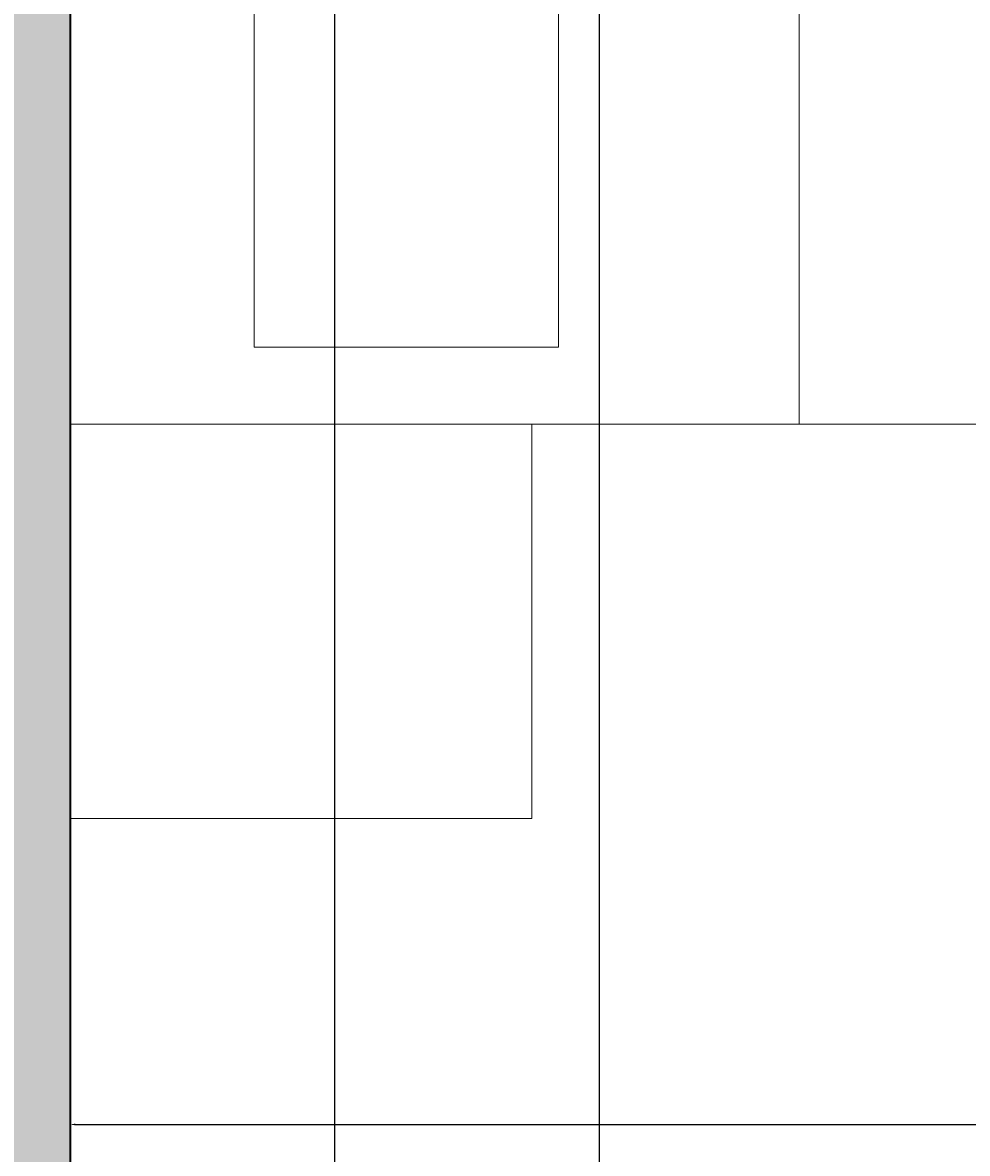
# Model space of a CAD drawing. Units: inches. Extents: x 1998 to 2588, y 1139 to 1977.
# Tile 64 of 134: x 2095 to 2127, y 1779 to 1817. Entities that reach past the tile are written whole.
import ezdxf

# ---------------------------------------------------------------- set-up
doc = ezdxf.new("R2010")
doc.units = ezdxf.units.IN
for name, color, linetype, lineweight in [('A-ANNO-DIMS', 2, 'Continuous', 18), ('A-WALL-PATT', 252, 'Continuous', 13), ('FUR', 21, 'Continuous', 18), ('WALL', 200, 'Continuous', 35)]:
    doc.layers.add(name, color=color, linetype=linetype, lineweight=lineweight)
doc.styles.get("Standard").update_dxf_attribs({"font": 'arial.ttf'})
doc.dimstyles.get("Standard").update_dxf_attribs({"dimtxt": 0.18, "dimasz": 0.18, "dimexe": 0.18, "dimexo": 0.0625, "dimgap": 0.09, "dimtad": 0, "dimtih": 1, "dimtoh": 1, "dimdec": 4, "dimzin": 0, "dimdsep": 46, "dimtxsty": 'Standard', "dimcen": 0.09, "dimadec": 0, "dimazin": 0, "dimtfac": 1, "dimtdec": 4, "dimtofl": 0, "dimtmove": 0, "dimatfit": 3, "dimfxl": 1, "dimtolj": 1, "dimtzin": 0, "dimarcsym": 0})

# ---------------------------------------------------------------- blocks, each defined once
blk = doc.blocks.new('BED-WITH-NIGHTSTANDS')
blk.add_line((24.799, 13.424), (24.799, 47.436))
for points in [[(0, 56), (65.221, 56), (65.221, 13.424), (0, 13.424)], [(6.254, 16.049), (16.605, 16.049), (16.605, 34.569), (6.254, 34.569)], [(0, 0), (15.699, 0), (15.699, 13.424), (0, 13.424)]]:
    blk.add_lwpolyline(points, close=True)
blk = doc.blocks.new('*D14')
at = {"layer": 'A-ANNO-DIMS', "color": 0, "lineweight": -2, "transparency": 16777216}
for p, q in [((2096.973, 1789.982), (2096.973, 1779.451)), ((2162.194, 1789.982), (2162.194, 1779.451)), ((2097.153, 1779.631), (2129.055, 1779.631)), ((2162.014, 1779.631), (2130.112, 1779.631))]:
    blk.add_line(p, q, dxfattribs=at)
at = {"layer": 'A-ANNO-DIMS', "color": 0, "transparency": 16777216}
for points in [[(2097.153, 1779.661), (2097.153, 1779.601), (2096.973, 1779.631)], [(2162.014, 1779.661), (2162.014, 1779.601), (2162.194, 1779.631)]]:
    blk.add_solid(points, dxfattribs=at)
at = {"layer": 'Defpoints', "color": 0, "transparency": 16777216}
for p in [(2096.973, 1790.045), (2162.194, 1790.045), (2162.194, 1779.631)]:
    blk.add_point(p, dxfattribs=at)
at = {"layer": 'A-ANNO-DIMS', "color": 0, "transparency": 16777216, "insert": (2129.584, 1779.631), "char_height": 0.18, "attachment_point": 5}
blk.add_mtext('\\A1;65 TYP.', dxfattribs=at)
blk = doc.blocks.new('*D40')
at = {"layer": 'A-ANNO-DIMS', "color": 0, "lineweight": -2, "transparency": 16777216}
for p, q in [((2105.973, 1628.541), (2105.973, 1977.362)), ((2114.973, 1628.804), (2114.973, 1977.362)), ((2106.153, 1977.182), (2110.324, 1977.182)), ((2114.793, 1977.182), (2110.622, 1977.182))]:
    blk.add_line(p, q, dxfattribs=at)
at = {"layer": 'A-ANNO-DIMS', "color": 0, "transparency": 16777216}
for points in [[(2106.153, 1977.212), (2106.153, 1977.152), (2105.973, 1977.182)], [(2114.793, 1977.212), (2114.793, 1977.152), (2114.973, 1977.182)]]:
    blk.add_solid(points, dxfattribs=at)
at = {"layer": 'Defpoints', "color": 0, "transparency": 16777216}
for p in [(2114.973, 1977.182), (2114.973, 1628.742), (2105.973, 1628.478)]:
    blk.add_point(p, dxfattribs=at)
at = {"layer": 'A-ANNO-DIMS', "color": 0, "transparency": 16777216, "insert": (2110.473, 1977.182), "char_height": 0.18, "attachment_point": 5}
blk.add_mtext('\\A1;9', dxfattribs=at)

msp = doc.modelspace()

# ---------------------------------------------------------------- hatches: boundary and pattern name
at = {"layer": 'A-WALL-PATT'}
h = msp.add_hatch(color=256, dxfattribs=at)
h.dxf.hatch_style = 1
h.paths.add_polyline_path([(2222.9729, 1888.7324), (2099.4125, 1888.7324), (2099.4125, 1879.7324), (2222.9729, 1879.7324)])
h.paths.add_polyline_path([(2096.9729, 1868.3278), (2087.9729, 1868.3278), (2087.9729, 1775.637), (2096.9729, 1775.637)])
h.paths.add_polyline_path([(2227.4729, 1868.3278), (2222.9729, 1868.3278), (2222.9729, 1774.3318), (2227.4729, 1774.3318)])
h.paths.add_polyline_path([(2188.3019, 1759.7324), (2138.6074, 1759.7324), (2099.4125, 1759.7324), (2099.4125, 1755.2324), (2176.9729, 1755.2324), (2188.3019, 1755.2324)])
h.paths.add_polyline_path([(2087.9729, 1759.7324), (2059.4729, 1759.7324), (2059.4729, 1702.7324), (2087.9729, 1702.7324), (2087.9729, 1707.2324), (2063.9729, 1707.2324), (2063.9729, 1755.2324), (2087.9729, 1755.2324)])
h.paths.add_polyline_path([(2096.9729, 1755.2324), (2087.9729, 1755.2324), (2087.9729, 1707.2324), (2096.9729, 1707.2324)])
h.paths.add_polyline_path([(2187.0461, 1707.2324), (2105.9729, 1707.2324), (2096.9729, 1707.2324), (2087.9729, 1707.2324), (2087.9729, 1702.7324), (2105.9729, 1702.7324), (2114.9729, 1702.7324), (2187.0461, 1702.7324)])
h.paths.add_polyline_path([(2181.4729, 1719.2028), (2176.9729, 1719.2028), (2176.9729, 1707.2324), (2181.4729, 1707.2324)])
h.paths.add_polyline_path([(2216.0332, 1588.7324), (2114.9729, 1588.7324), (2105.9729, 1588.7324), (2105.9729, 1584.2324), (2216.0332, 1584.2324)])
h.paths.add_polyline_path([(2077.691, 1588.7324), (2061.4729, 1588.7324), (2061.4729, 1584.2324), (2077.691, 1584.2324)])
h.paths.add_polyline_path([(2105.9729, 1588.7324), (2098.0956, 1588.7324), (2098.0956, 1584.2324), (2105.9729, 1584.2324)])
h.paths.add_polyline_path([(2114.9729, 1596.2642), (2110.1012, 1596.2642), (2105.9729, 1596.2642), (2105.9729, 1588.7324), (2114.9729, 1588.7324)])
h.paths.add_polyline_path([(2114.9729, 1584.2324), (2105.9729, 1584.2324), (2105.9729, 1580.249), (2110.1012, 1580.249), (2114.9729, 1580.249)])
h.paths.add_polyline_path([(2114.9729, 1547.7716), (2110.1012, 1547.7716, -0.0318759), (2105.9729, 1548.035), (2105.9729, 1470.2324), (2108.3775, 1470.2324), (2108.3775, 1465.7324), (2186.2943, 1465.7324), (2186.2943, 1470.2324), (2114.9729, 1470.2324)])
h.paths.add_polyline_path([(2227.4729, 1584.2324), (2222.9729, 1584.2324), (2222.9729, 1486.137), (2227.4729, 1486.137)])
h.paths.add_polyline_path([(2295.4138, 1593.2324), (2227.4729, 1593.2324), (2227.4729, 1588.7324), (2295.4138, 1588.7324), (2295.4138, 1591.8729)])
h.paths.add_polyline_path([(2345.9729, 1627.1165), (2341.4729, 1627.1165), (2341.4729, 1593.2324), (2337.2869, 1593.2324), (2337.2869, 1591.8729), (2337.2869, 1588.7324), (2345.9729, 1588.7324)])
h.paths.add_polyline_path([(2291.9729, 1588.7324), (2287.4729, 1588.7324), (2287.4729, 1522.7324), (2291.9729, 1522.7324)])
h.paths.add_polyline_path([(2291.9729, 1522.7324), (2287.4729, 1522.7324), (2227.4729, 1522.7324), (2227.4729, 1518.2324), (2291.9729, 1518.2324)])
h.paths.add_polyline_path([(2295.7347, 1519.5919), (2295.7347, 1522.7324), (2291.9729, 1522.7324), (2291.9729, 1518.2324), (2295.7347, 1518.2324)])
h.paths.add_polyline_path([(2345.9729, 1522.7324), (2337.6078, 1522.7324), (2337.6078, 1519.5919), (2337.6078, 1518.2324), (2341.4729, 1518.2324), (2341.4729, 1488.5616), (2345.9729, 1488.5616)])
h.paths.add_polyline_path([(2345.9729, 1468.1569), (2341.4729, 1468.1569), (2341.4729, 1374.2324), (2227.4729, 1374.2324), (2227.4729, 1369.7324), (2345.9729, 1369.7324)])
h.paths.add_polyline_path([(2345.9729, 1369.7324), (2341.4729, 1369.7324), (2341.4729, 1362.2324), (2345.9729, 1362.2324)])
h.paths.add_polyline_path([(2345.9729, 1317.7324), (2345.9729, 1322.2324), (2341.4729, 1322.2324), (2341.4729, 1285.137), (2345.9729, 1285.137)], flags=17)
h.paths.add_polyline_path([(2356.2096, 1322.2324), (2345.9729, 1322.2324), (2345.9729, 1317.7324), (2356.2096, 1317.7324), (2356.2096, 1319.3088)], flags=17)
h.paths.add_polyline_path([(2393.9729, 1322.2324), (2375.6999, 1322.2324), (2375.6999, 1319.3088, -0.0202458), (2375.636, 1317.7324), (2393.9729, 1317.7324)], flags=17)
h.paths.add_polyline_path([(2398.4729, 1322.2324), (2393.9729, 1322.2324), (2393.9729, 1317.7324), (2393.9729, 1237.7324), (2345.9729, 1237.7324), (2345.9729, 1264.7324), (2341.4729, 1264.7324), (2341.4729, 1228.7324), (2393.9729, 1228.7324), (2482.7412, 1228.7324), (2482.7412, 1237.7324), (2398.4729, 1237.7324), (2398.4729, 1297.1029)])
h.paths.add_polyline_path([(2398.4729, 1362.2324), (2393.9729, 1362.2324), (2393.9729, 1357.7324), (2398.4729, 1357.7324)])
h.paths.add_polyline_path([(2345.9729, 1329.7549), (2341.4729, 1329.7549), (2341.4729, 1322.2324), (2345.9729, 1322.2324)])

# ---------------------------------------------------------------- linework, layer by layer
at = {"layer": 'WALL'}
msp.add_line((2096.9729, 1868.3278), (2096.9729, 1775.637), dxfattribs=at)

# ---------------------------------------------------------------- block references
at = {"layer": 'FUR'}
msp.add_blockref('BED-WITH-NIGHTSTANDS', (2096.973, 1790.045), dxfattribs=at)

# ---------------------------------------------------------------- dimensions: what is measured, and where the dimension line sits
at = {"layer": 'A-ANNO-DIMS'}
dim = msp.add_linear_dim(base=(2114.9729, 1977.1824), p1=(2105.9729, 1628.4781), p2=(2114.9729, 1628.7416), dimstyle='Standard', override={"dimdec": 0, "dimlfac": 1, "dimrnd": 0, "dimzin": 0, "dimdsep": 46, "dimlunit": 2}, dxfattribs=at)
dim.commit()
dim.dimension.update_dxf_attribs({"geometry": '*D40', "text_midpoint": (2110.4729, 1977.1824)})
dim = msp.add_linear_dim(base=(2162.1944, 1779.6308), p1=(2096.9729, 1790.0445), p2=(2162.1944, 1790.0445), text='<> TYP.', dimstyle='Standard', override={"dimdec": 0, "dimlfac": 1, "dimrnd": 0, "dimzin": 0, "dimdsep": 46, "dimlunit": 2}, dxfattribs=at)
dim.commit()
dim.dimension.update_dxf_attribs({"geometry": '*D14', "text_midpoint": (2129.5836, 1779.6308)})

doc.saveas('drawing.dxf')
